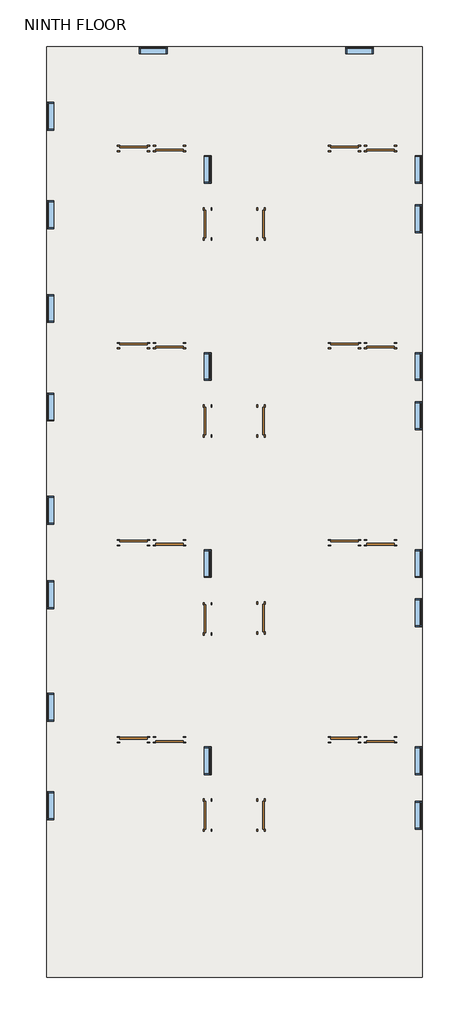
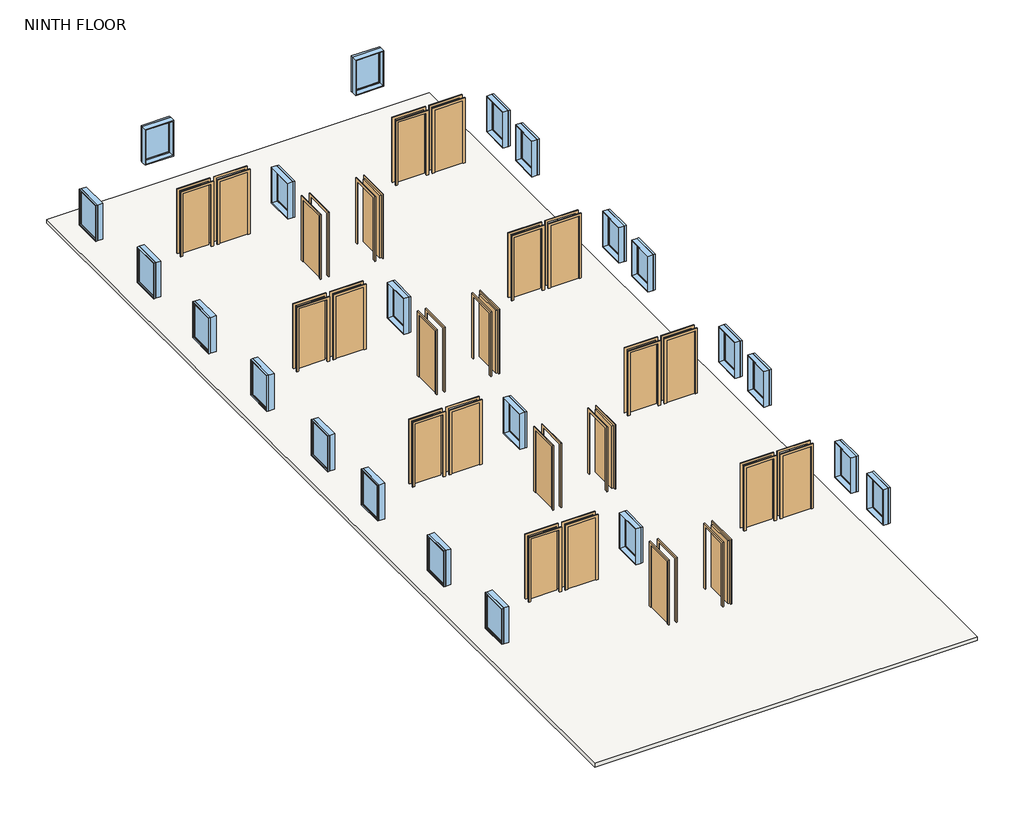
# One storey: 24 doors, 22 windows, 1 slab.
"""IFC4 building model written with IfcOpenShell, lengths in millimetres."""

from ifc_helpers import new_model, si_unit, frame, origin, place, context, project, spatial, polyline, outline, extrude, transform, mapped, element, save
from components import door_686f89d2, door_16372e1c, door_a90ba1ad, door_0ca8825f, window_c1f32544

model = new_model("IFC4")

# Units and contexts
model_context = context("Model", 3, world=origin())
ifc_project = project(units=[si_unit("LENGTHUNIT", "METRE", prefix="MILLI")], contexts=[model_context])

# Site, building, storey
site = spatial("IfcSite", under=ifc_project)
building = spatial("IfcBuilding", under=site)
storey = spatial("IfcBuildingStorey", under=building, Name="NINTH FLOOR", Elevation=28803.6)

# Doors
placement = place(None, origin())
door_shape = door_686f89d2(model_context)
element("IfcDoor", 1, ObjectType="Single-Flush : 36\" x 84\"", at=placement, inside=storey, context=model_context, shape_type="MappedRepresentation", body=[
    mapped(door_shape, transform((-9863.5902461, 11952.2710592, 28803.6), x_axis=(-1.0, 0.0, 0.0), y_axis=(0.0, -1.0, 0.0), z_axis=(0.0, 0.0, 1.0))),
])
element("IfcDoor", 2, ObjectType="Single-Flush : 36\" x 84\"", at=placement, inside=storey, context=model_context, shape_type="MappedRepresentation", body=[
    mapped(door_shape, transform((-2929.3902461, 11952.2710592, 28803.6), x_axis=(-1.0, 0.0, 0.0), y_axis=(0.0, -1.0, 0.0), z_axis=(0.0, 0.0, 1.0))),
])
element("IfcDoor", 3, ObjectType="Single-Flush : 36\" x 84\"", at=placement, inside=storey, context=model_context, shape_type="MappedRepresentation", body=[
    mapped(door_shape, transform((-9863.5902461, 5475.2710592, 28803.6), x_axis=(-1.0, 0.0, 0.0), y_axis=(0.0, -1.0, 0.0), z_axis=(0.0, 0.0, 1.0))),
])
element("IfcDoor", 4, ObjectType="Single-Flush : 36\" x 84\"", at=placement, inside=storey, context=model_context, shape_type="MappedRepresentation", body=[
    mapped(door_shape, transform((-2929.3902461, 5475.2710592, 28803.6), x_axis=(-1.0, 0.0, 0.0), y_axis=(0.0, -1.0, 0.0), z_axis=(0.0, 0.0, 1.0))),
])
element("IfcDoor", 5, ObjectType="Single-Flush : 36\" x 84\"", at=placement, inside=storey, context=model_context, shape_type="MappedRepresentation", body=[
    mapped(door_shape, transform((-9863.5902461, -1001.7289408, 28803.6), x_axis=(-1.0, 0.0, 0.0), y_axis=(0.0, -1.0, 0.0), z_axis=(0.0, 0.0, 1.0))),
])
element("IfcDoor", 6, ObjectType="Single-Flush : 36\" x 84\"", at=placement, inside=storey, context=model_context, shape_type="MappedRepresentation", body=[
    mapped(door_shape, transform((-2929.3902461, -1001.7289408, 28803.6), x_axis=(-1.0, 0.0, 0.0), y_axis=(0.0, -1.0, 0.0), z_axis=(0.0, 0.0, 1.0))),
])
element("IfcDoor", 7, ObjectType="Single-Flush : 36\" x 84\"", at=placement, inside=storey, context=model_context, shape_type="MappedRepresentation", body=[
    mapped(door_shape, transform((-9863.5902461, -7478.7289408, 28803.6), x_axis=(-1.0, 0.0, 0.0), y_axis=(0.0, -1.0, 0.0), z_axis=(0.0, 0.0, 1.0))),
])
element("IfcDoor", 8, ObjectType="Single-Flush : 36\" x 84\"", at=placement, inside=storey, context=model_context, shape_type="MappedRepresentation", body=[
    mapped(door_shape, transform((-2929.3902461, -7478.7289408, 28803.6), x_axis=(-1.0, 0.0, 0.0), y_axis=(0.0, -1.0, 0.0), z_axis=(0.0, 0.0, 1.0))),
])
door_2_shape = door_16372e1c(model_context)
element("IfcDoor", 9, ObjectType="Single-Flush : 36\" x 84\"", at=placement, inside=storey, context=model_context, shape_type="MappedRepresentation", body=[
    mapped(door_2_shape, transform((-8682.4902461, 11952.2710592, 28803.6), x_axis=(-1.0, 0.0, 0.0), y_axis=(0.0, -1.0, 0.0), z_axis=(0.0, 0.0, 1.0))),
])
element("IfcDoor", 10, ObjectType="Single-Flush : 36\" x 84\"", at=placement, inside=storey, context=model_context, shape_type="MappedRepresentation", body=[
    mapped(door_2_shape, transform((-1748.2902461, 11952.2710592, 28803.6), x_axis=(-1.0, 0.0, 0.0), y_axis=(0.0, -1.0, 0.0), z_axis=(0.0, 0.0, 1.0))),
])
element("IfcDoor", 11, ObjectType="Single-Flush : 36\" x 84\"", at=placement, inside=storey, context=model_context, shape_type="MappedRepresentation", body=[
    mapped(door_2_shape, transform((-8682.4902461, 5475.2710592, 28803.6), x_axis=(-1.0, 0.0, 0.0), y_axis=(0.0, -1.0, 0.0), z_axis=(0.0, 0.0, 1.0))),
])
element("IfcDoor", 12, ObjectType="Single-Flush : 36\" x 84\"", at=placement, inside=storey, context=model_context, shape_type="MappedRepresentation", body=[
    mapped(door_2_shape, transform((-1748.2902461, 5475.2710592, 28803.6), x_axis=(-1.0, 0.0, 0.0), y_axis=(0.0, -1.0, 0.0), z_axis=(0.0, 0.0, 1.0))),
])
element("IfcDoor", 13, ObjectType="Single-Flush : 36\" x 84\"", at=placement, inside=storey, context=model_context, shape_type="MappedRepresentation", body=[
    mapped(door_2_shape, transform((-8682.4902461, -1001.7289408, 28803.6), x_axis=(-1.0, 0.0, 0.0), y_axis=(0.0, -1.0, 0.0), z_axis=(0.0, 0.0, 1.0))),
])
element("IfcDoor", 14, ObjectType="Single-Flush : 36\" x 84\"", at=placement, inside=storey, context=model_context, shape_type="MappedRepresentation", body=[
    mapped(door_2_shape, transform((-1748.2902461, -1001.7289408, 28803.6), x_axis=(-1.0, 0.0, 0.0), y_axis=(0.0, -1.0, 0.0), z_axis=(0.0, 0.0, 1.0))),
])
element("IfcDoor", 15, ObjectType="Single-Flush : 36\" x 84\"", at=placement, inside=storey, context=model_context, shape_type="MappedRepresentation", body=[
    mapped(door_2_shape, transform((-8682.4902461, -7478.7289408, 28803.6), x_axis=(-1.0, 0.0, 0.0), y_axis=(0.0, -1.0, 0.0), z_axis=(0.0, 0.0, 1.0))),
])
element("IfcDoor", 16, ObjectType="Single-Flush : 36\" x 84\"", at=placement, inside=storey, context=model_context, shape_type="MappedRepresentation", body=[
    mapped(door_2_shape, transform((-1748.2902461, -7478.7289408, 28803.6), x_axis=(-1.0, 0.0, 0.0), y_axis=(0.0, -1.0, 0.0), z_axis=(0.0, 0.0, 1.0))),
])
door_3_shape = door_a90ba1ad(model_context)
element("IfcDoor", 17, ObjectType="Single-Flush : 36\" x 84\"", at=placement, inside=storey, context=model_context, shape_type="MappedRepresentation", body=[
    mapped(door_3_shape, transform((-7425.1902461, 9475.7710592, 28803.6), x_axis=(0.0, -1.0, 0.0), y_axis=(1.0, 0.0, 0.0), z_axis=(0.0, 0.0, 1.0))),
])
element("IfcDoor", 18, ObjectType="Single-Flush : 36\" x 84\"", at=placement, inside=storey, context=model_context, shape_type="MappedRepresentation", body=[
    mapped(door_3_shape, transform((-7425.1902461, 2998.7710592, 28803.6), x_axis=(0.0, -1.0, 0.0), y_axis=(1.0, 0.0, 0.0), z_axis=(0.0, 0.0, 1.0))),
])
element("IfcDoor", 19, ObjectType="Single-Flush : 36\" x 84\"", at=placement, inside=storey, context=model_context, shape_type="MappedRepresentation", body=[
    mapped(door_3_shape, transform((-7425.1902461, -9955.2289408, 28803.6), x_axis=(0.0, -1.0, 0.0), y_axis=(1.0, 0.0, 0.0), z_axis=(0.0, 0.0, 1.0))),
])
element("IfcDoor", 20, ObjectType="Single-Flush : 36\" x 84\"", at=placement, inside=storey, context=model_context, shape_type="MappedRepresentation", body=[
    mapped(door_3_shape, transform((-7425.1902461, -3503.6289408, 28803.6), x_axis=(0.0, -1.0, 0.0), y_axis=(1.0, 0.0, 0.0), z_axis=(0.0, 0.0, 1.0))),
])
door_4_shape = door_0ca8825f(model_context)
element("IfcDoor", 21, ObjectType="Single-Flush : 36\" x 84\"", at=placement, inside=storey, context=model_context, shape_type="MappedRepresentation", body=[
    mapped(door_4_shape, transform((-5672.5902461, 9475.7710592, 28803.6), x_axis=(0.0, -1.0, 0.0), y_axis=(1.0, 0.0, 0.0), z_axis=(0.0, 0.0, 1.0))),
])
element("IfcDoor", 22, ObjectType="Single-Flush : 36\" x 84\"", at=placement, inside=storey, context=model_context, shape_type="MappedRepresentation", body=[
    mapped(door_4_shape, transform((-5672.5902461, 2998.7710592, 28803.6), x_axis=(0.0, -1.0, 0.0), y_axis=(1.0, 0.0, 0.0), z_axis=(0.0, 0.0, 1.0))),
])
element("IfcDoor", 23, ObjectType="Single-Flush : 36\" x 84\"", at=placement, inside=storey, context=model_context, shape_type="MappedRepresentation", body=[
    mapped(door_4_shape, transform((-5672.5902461, -9955.2289408, 28803.6), x_axis=(0.0, -1.0, 0.0), y_axis=(1.0, 0.0, 0.0), z_axis=(0.0, 0.0, 1.0))),
])
element("IfcDoor", 24, ObjectType="Single-Flush : 36\" x 84\"", at=placement, inside=storey, context=model_context, shape_type="MappedRepresentation", body=[
    mapped(door_4_shape, transform((-5672.5902461, -3478.2289408, 28803.6), x_axis=(0.0, -1.0, 0.0), y_axis=(1.0, 0.0, 0.0), z_axis=(0.0, 0.0, 1.0))),
])

# Slab
element("IfcSlab", 25, ObjectType="Generic - 12\"", at=placement, inside=storey, context=model_context, shape_type="SweptSolid", body=[
    extrude(outline(polyline([(-376.6902461, 15305.0710592), (-376.6902461, -15289.2289408), (-12721.0902461, -15289.2289408), (-12721.0902461, 15305.0710592), (-376.6902461, 15305.0710592)])), frame((0.0, 0.0, 28676.6), z_axis=(0.0, 0.0, 1.0), x_axis=(1.0, 0.0, 0.0)), (0.0, 0.0, 1.0), 127.0),
])

# Windows
window_shape = window_c1f32544(model_context)
element("IfcWindow", 26, ObjectType="Fixed : 36\" x 48\"", at=placement, inside=storey, context=model_context, shape_type="MappedRepresentation", body=[
    mapped(window_shape, transform((-9177.7902461, 15190.7710592, 28803.6), x_axis=(1.0, 0.0, 0.0), y_axis=(0.0, 1.0, 0.0), z_axis=(0.0, 0.0, 1.0))),
])
element("IfcWindow", 27, ObjectType="Fixed : 36\" x 48\"", at=placement, inside=storey, context=model_context, shape_type="MappedRepresentation", body=[
    mapped(window_shape, transform((-2395.9902461, 15190.7710592, 28803.6), x_axis=(1.0, 0.0, 0.0), y_axis=(0.0, 1.0, 0.0), z_axis=(0.0, 0.0, 1.0))),
])
element("IfcWindow", 28, ObjectType="Fixed : 36\" x 48\"", at=placement, inside=storey, context=model_context, shape_type="MappedRepresentation", body=[
    mapped(window_shape, transform((-490.9902461, 11228.3710592, 28803.6), x_axis=(0.0, -1.0, 0.0), y_axis=(1.0, 0.0, 0.0), z_axis=(0.0, 0.0, 1.0))),
])
element("IfcWindow", 29, ObjectType="Fixed : 36\" x 48\"", at=placement, inside=storey, context=model_context, shape_type="MappedRepresentation", body=[
    mapped(window_shape, transform((-490.9902461, 9609.1210592, 28803.6), x_axis=(0.0, -1.0, 0.0), y_axis=(1.0, 0.0, 0.0), z_axis=(0.0, 0.0, 1.0))),
])
element("IfcWindow", 30, ObjectType="Fixed : 36\" x 48\"", at=placement, inside=storey, context=model_context, shape_type="MappedRepresentation", body=[
    mapped(window_shape, transform((-490.9902461, 4751.3710592, 28803.6), x_axis=(0.0, -1.0, 0.0), y_axis=(1.0, 0.0, 0.0), z_axis=(0.0, 0.0, 1.0))),
])
element("IfcWindow", 31, ObjectType="Fixed : 36\" x 48\"", at=placement, inside=storey, context=model_context, shape_type="MappedRepresentation", body=[
    mapped(window_shape, transform((-490.9902461, 3132.1210592, 28803.6), x_axis=(0.0, -1.0, 0.0), y_axis=(1.0, 0.0, 0.0), z_axis=(0.0, 0.0, 1.0))),
])
element("IfcWindow", 32, ObjectType="Fixed : 36\" x 48\"", at=placement, inside=storey, context=model_context, shape_type="MappedRepresentation", body=[
    mapped(window_shape, transform((-490.9902461, -1725.6289408, 28803.6), x_axis=(0.0, -1.0, 0.0), y_axis=(1.0, 0.0, 0.0), z_axis=(0.0, 0.0, 1.0))),
])
element("IfcWindow", 33, ObjectType="Fixed : 36\" x 48\"", at=placement, inside=storey, context=model_context, shape_type="MappedRepresentation", body=[
    mapped(window_shape, transform((-490.9902461, -3344.8789408, 28803.6), x_axis=(0.0, -1.0, 0.0), y_axis=(1.0, 0.0, 0.0), z_axis=(0.0, 0.0, 1.0))),
])
element("IfcWindow", 34, ObjectType="Fixed : 36\" x 48\"", at=placement, inside=storey, context=model_context, shape_type="MappedRepresentation", body=[
    mapped(window_shape, transform((-490.9902461, -8202.6289408, 28803.6), x_axis=(0.0, -1.0, 0.0), y_axis=(1.0, 0.0, 0.0), z_axis=(0.0, 0.0, 1.0))),
])
element("IfcWindow", 35, ObjectType="Fixed : 36\" x 48\"", at=placement, inside=storey, context=model_context, shape_type="MappedRepresentation", body=[
    mapped(window_shape, transform((-490.9902461, -9993.3289408, 28803.6), x_axis=(0.0, -1.0, 0.0), y_axis=(1.0, 0.0, 0.0), z_axis=(0.0, 0.0, 1.0))),
])
element("IfcWindow", 36, ObjectType="Fixed : 36\" x 48\"", at=placement, inside=storey, context=model_context, shape_type="MappedRepresentation", body=[
    mapped(window_shape, transform((-12606.7902461, -9612.3289408, 28803.6), x_axis=(0.0, 1.0, 0.0), y_axis=(-1.0, 0.0, 0.0), z_axis=(0.0, 0.0, 1.0))),
])
element("IfcWindow", 37, ObjectType="Fixed : 36\" x 48\"", at=placement, inside=storey, context=model_context, shape_type="MappedRepresentation", body=[
    mapped(window_shape, transform((-12606.7902461, -6373.8289408, 28803.6), x_axis=(0.0, 1.0, 0.0), y_axis=(-1.0, 0.0, 0.0), z_axis=(0.0, 0.0, 1.0))),
])
element("IfcWindow", 38, ObjectType="Fixed : 36\" x 48\"", at=placement, inside=storey, context=model_context, shape_type="MappedRepresentation", body=[
    mapped(window_shape, transform((-12606.7902461, -2678.1289408, 28803.6), x_axis=(0.0, 1.0, 0.0), y_axis=(-1.0, 0.0, 0.0), z_axis=(0.0, 0.0, 1.0))),
])
element("IfcWindow", 39, ObjectType="Fixed : 36\" x 48\"", at=placement, inside=storey, context=model_context, shape_type="MappedRepresentation", body=[
    mapped(window_shape, transform((-12606.7902461, 103.1710592, 28803.6), x_axis=(0.0, 1.0, 0.0), y_axis=(-1.0, 0.0, 0.0), z_axis=(0.0, 0.0, 1.0))),
])
element("IfcWindow", 40, ObjectType="Fixed : 36\" x 48\"", at=placement, inside=storey, context=model_context, shape_type="MappedRepresentation", body=[
    mapped(window_shape, transform((-12606.7902461, 3494.0710592, 28803.6), x_axis=(0.0, 1.0, 0.0), y_axis=(-1.0, 0.0, 0.0), z_axis=(0.0, 0.0, 1.0))),
])
element("IfcWindow", 41, ObjectType="Fixed : 36\" x 48\"", at=placement, inside=storey, context=model_context, shape_type="MappedRepresentation", body=[
    mapped(window_shape, transform((-12606.7902461, 6732.5710592, 28803.6), x_axis=(0.0, 1.0, 0.0), y_axis=(-1.0, 0.0, 0.0), z_axis=(0.0, 0.0, 1.0))),
])
element("IfcWindow", 42, ObjectType="Fixed : 36\" x 48\"", at=placement, inside=storey, context=model_context, shape_type="MappedRepresentation", body=[
    mapped(window_shape, transform((-12606.7902461, 9818.6710592, 28803.6), x_axis=(0.0, 1.0, 0.0), y_axis=(-1.0, 0.0, 0.0), z_axis=(0.0, 0.0, 1.0))),
])
element("IfcWindow", 43, ObjectType="Fixed : 36\" x 48\"", at=placement, inside=storey, context=model_context, shape_type="MappedRepresentation", body=[
    mapped(window_shape, transform((-12606.7902461, 13057.1710592, 28803.6), x_axis=(0.0, 1.0, 0.0), y_axis=(-1.0, 0.0, 0.0), z_axis=(0.0, 0.0, 1.0))),
])
element("IfcWindow", 44, ObjectType="Fixed : 36\" x 48\"", at=placement, inside=storey, context=model_context, shape_type="MappedRepresentation", body=[
    mapped(window_shape, transform((-7425.1902461, 11228.3710592, 28803.6), x_axis=(0.0, -1.0, 0.0), y_axis=(1.0, 0.0, 0.0), z_axis=(0.0, 0.0, 1.0))),
])
element("IfcWindow", 45, ObjectType="Fixed : 36\" x 48\"", at=placement, inside=storey, context=model_context, shape_type="MappedRepresentation", body=[
    mapped(window_shape, transform((-7425.1902461, 4751.3710592, 28803.6), x_axis=(0.0, -1.0, 0.0), y_axis=(1.0, 0.0, 0.0), z_axis=(0.0, 0.0, 1.0))),
])
element("IfcWindow", 46, ObjectType="Fixed : 36\" x 48\"", at=placement, inside=storey, context=model_context, shape_type="MappedRepresentation", body=[
    mapped(window_shape, transform((-7425.1902461, -1725.6289408, 28803.6), x_axis=(0.0, -1.0, 0.0), y_axis=(1.0, 0.0, 0.0), z_axis=(0.0, 0.0, 1.0))),
])
element("IfcWindow", 47, ObjectType="Fixed : 36\" x 48\"", at=placement, inside=storey, context=model_context, shape_type="MappedRepresentation", body=[
    mapped(window_shape, transform((-7425.1902461, -8202.6289408, 28803.6), x_axis=(0.0, -1.0, 0.0), y_axis=(1.0, 0.0, 0.0), z_axis=(0.0, 0.0, 1.0))),
])

save(model, "model.ifc")

# Revit data of these elements
# Type "Single-Flush : 36\" x 84\""
#   Type Mark = "1"
#   Construction Type Id = "MDOOR"
#   Assembly Code = "C1020"
#   Analytic Construction = "Metal"
#   Thickness = 0' - 2"
#   Heat Transfer Coefficient (U) = 0.651978 BTU/(h·ft²·°F)
#   Height = 7' - 0"
#   Trim Projection Ext = 0' - 1"
#   Trim Projection Int = 0' - 1"
#   Trim Width = 0' - 3"
#   Width = 3' - 0"
#   Define Thermal Properties by = 1
#   Door Material = Door - Panel
#   Frame Material = Door - Frame
#   Visual Light Transmittance = 0
#   Solar Heat Gain Coefficient = 0
#   Function = (empty or 0)
#   Wall Closure = (empty or 0)
# Type "Generic - 12\""
#   Assembly Code = "B1010"
#   Function = 0
#   Layers, outside or top first: 0' - 5" no material (function 1)
# Type "Fixed : 36\" x 48\""
#   Type Mark = "1"
#   Construction Type Id = "GSP4R"
#   Assembly Code = "B2020100"
#   Analytic Construction = "1/8 in Pilkington single glazing"
#   Visual Light Transmittance = 0.9
#   Solar Heat Gain Coefficient = 0.78
#   Heat Transfer Coefficient (U) = 0.6496 BTU/(h·ft²·°F)
#   Height = 4' - 0"
#   Default Sill Height = 3' - 0"
#   Width = 3' - 0"
#   Window Inset = 0' - 0 3/4"
#   Define Thermal Properties by = 1
#   Glass Pane Material = Glass
#   Sash Material = Sash
#   Wall Closure = (empty or 0)
# Elements 1, 2, 3, 4, 5, 6, 7, 8, 9, 10, 11, 12, 13, 14, 15, 16, 17, 18, 19, 20, 21, 22, 23, 24 (IfcDoor, "Single-Flush : 36\" x 84\"")
#   Phase Created = New Construction
#   Materials on its faces: "Door - Frame", "Door - Panel"
# Element 25 (IfcSlab, "Generic - 12\"")
#   Height Offset From Level = 0' - 0"
#   Phase Created = New Construction
#   Materials on its faces: "Default Floor"
# Element 26 (IfcWindow, "Fixed : 36\" x 48\"")
#   Mark = "205"
#   Phase Created = New Construction
#   Materials on its faces: "Sash", "Glass"
# Element 27 (IfcWindow, "Fixed : 36\" x 48\"")
#   Mark = "206"
#   Phase Created = New Construction
#   Materials on its faces: "Sash", "Glass"
# Element 28 (IfcWindow, "Fixed : 36\" x 48\"")
#   Mark = "207"
#   Phase Created = New Construction
#   Materials on its faces: "Sash", "Glass"
# Element 29 (IfcWindow, "Fixed : 36\" x 48\"")
#   Mark = "208"
#   Phase Created = New Construction
#   Materials on its faces: "Sash", "Glass"
# Element 30 (IfcWindow, "Fixed : 36\" x 48\"")
#   Mark = "209"
#   Phase Created = New Construction
#   Materials on its faces: "Sash", "Glass"
# Element 31 (IfcWindow, "Fixed : 36\" x 48\"")
#   Mark = "210"
#   Phase Created = New Construction
#   Materials on its faces: "Sash", "Glass"
# Element 32 (IfcWindow, "Fixed : 36\" x 48\"")
#   Mark = "211"
#   Phase Created = New Construction
#   Materials on its faces: "Sash", "Glass"
# Element 33 (IfcWindow, "Fixed : 36\" x 48\"")
#   Mark = "212"
#   Phase Created = New Construction
#   Materials on its faces: "Sash", "Glass"
# Element 34 (IfcWindow, "Fixed : 36\" x 48\"")
#   Mark = "213"
#   Phase Created = New Construction
#   Materials on its faces: "Sash", "Glass"
# Element 35 (IfcWindow, "Fixed : 36\" x 48\"")
#   Mark = "214"
#   Phase Created = New Construction
#   Materials on its faces: "Sash", "Glass"
# Element 36 (IfcWindow, "Fixed : 36\" x 48\"")
#   Mark = "215"
#   Phase Created = New Construction
#   Materials on its faces: "Sash", "Glass"
# Element 37 (IfcWindow, "Fixed : 36\" x 48\"")
#   Mark = "216"
#   Phase Created = New Construction
#   Materials on its faces: "Sash", "Glass"
# Element 38 (IfcWindow, "Fixed : 36\" x 48\"")
#   Mark = "217"
#   Phase Created = New Construction
#   Materials on its faces: "Sash", "Glass"
# Element 39 (IfcWindow, "Fixed : 36\" x 48\"")
#   Mark = "218"
#   Phase Created = New Construction
#   Materials on its faces: "Sash", "Glass"
# Element 40 (IfcWindow, "Fixed : 36\" x 48\"")
#   Mark = "219"
#   Phase Created = New Construction
#   Materials on its faces: "Sash", "Glass"
# Element 41 (IfcWindow, "Fixed : 36\" x 48\"")
#   Mark = "220"
#   Phase Created = New Construction
#   Materials on its faces: "Sash", "Glass"
# Element 42 (IfcWindow, "Fixed : 36\" x 48\"")
#   Mark = "221"
#   Phase Created = New Construction
#   Materials on its faces: "Sash", "Glass"
# Element 43 (IfcWindow, "Fixed : 36\" x 48\"")
#   Mark = "222"
#   Phase Created = New Construction
#   Materials on its faces: "Sash", "Glass"
# Element 44 (IfcWindow, "Fixed : 36\" x 48\"")
#   Mark = "223"
#   Phase Created = New Construction
#   Materials on its faces: "Sash", "Glass"
# Element 45 (IfcWindow, "Fixed : 36\" x 48\"")
#   Mark = "224"
#   Phase Created = New Construction
#   Materials on its faces: "Sash", "Glass"
# Element 46 (IfcWindow, "Fixed : 36\" x 48\"")
#   Mark = "225"
#   Phase Created = New Construction
#   Materials on its faces: "Sash", "Glass"
# Element 47 (IfcWindow, "Fixed : 36\" x 48\"")
#   Mark = "226"
#   Phase Created = New Construction
#   Materials on its faces: "Sash", "Glass"
# Materials
#   "Door - Panel": class "Wood", colour RGB 210 159 95, transparency 0
#   "Door - Frame": colour RGB 118 70 51, transparency 0
#   "Glass": class "Glass", colour RGB 0 128 192, transparency 0.75, Description = "Soda Lime Glass", Cost = 0
#   "Sash": class "Wood", colour RGB 224 178 126, transparency 0
#   "Default Floor": colour RGB 128 128 128, transparency 0
